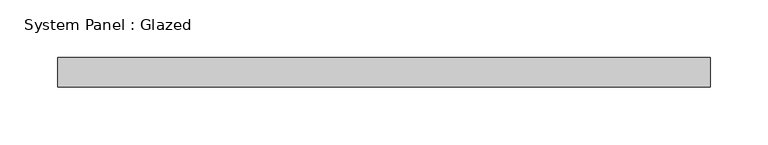
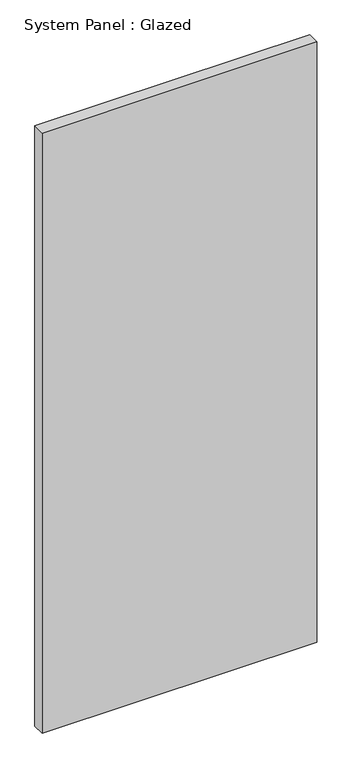
"""IFC4 building model written with IfcOpenShell, lengths in millimetres: plate geometry, System Panel : Glazed."""

from ifc_helpers import new_model, si_unit, origin, origin_with_axes, place, context, project, spatial, polyline, outline, extrude, source, transform, mapped, element, save


def system_panel_glazed_a7448bf8(model_context):
    return source(origin(), model_context, "Body", "SweptSolid", [
        extrude(outline(polyline([(282.575, 19.05), (-282.575, 19.05), (-282.575, 44.45), (282.575, 44.45), (282.575, 19.05)])), origin_with_axes(), (0.0, 0.0, 1.0), 1304.017105),
    ])


if __name__ == "__main__":
    model = new_model("IFC4")
    model_context = context("Model", 3, world=origin())
    ifc_project = project(units=[si_unit("LENGTHUNIT", "METRE", prefix="MILLI")], contexts=[model_context])
    site = spatial("IfcSite", under=ifc_project)
    building = spatial("IfcBuilding", under=site)
    placement = place(None, origin())
    system_panel_glazed_shape = system_panel_glazed_a7448bf8(model_context)
    element("IfcPlate", 1, ObjectType="System Panel : Glazed", at=placement, inside=building, context=model_context, shape_type="MappedRepresentation", body=[
        mapped(system_panel_glazed_shape, transform((0.0, 0.0, 0.0), x_axis=(1.0, 0.0, 0.0), y_axis=(0.0, 1.0, 0.0), z_axis=(0.0, 0.0, 1.0))),
    ])
    save(model, "model.ifc")

# Revit data of these elements
# Type "System Panel : Glazed"
#   Construction Type Id = "GSP4R"
#   Analytic Construction = "1/8 in Pilkington single glazing"
#   Visual Light Transmittance = 0.9
#   Solar Heat Gain Coefficient = 0.86
#   Heat Transfer Coefficient (U) = 1.18115 BTU/(h·ft²·°F)
#   Define Thermal Properties by = 1
# Element 1 (IfcPlate, "System Panel : Glazed")
#   Materials on its faces: "Glass"
# Materials
#   "Glass": class "Glass", colour RGB 0 128 192, transparency 0.75, Description = "Soda Lime Glass", Cost = 0
